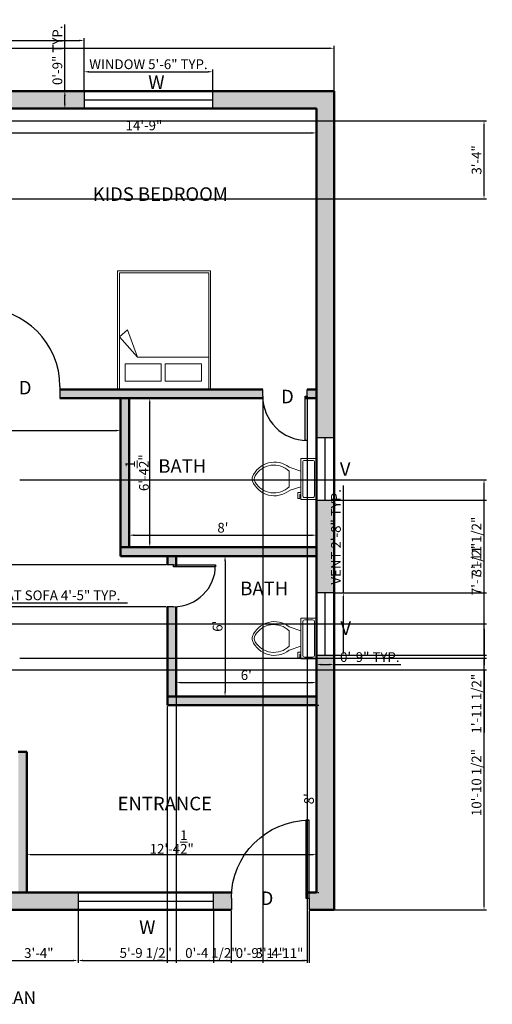
# Model space of a CAD drawing. Units: inches. Extents: x 2168 to 2706, y 2255 to 2760.
# Tile 4 of 4: x 2463 to 2706, y 2255 to 2760. Entities that reach past the tile are written whole.
import ezdxf

# ---------------------------------------------------------------- set-up
doc = ezdxf.new("R2010")
doc.units = ezdxf.units.IN
for name, color, linetype, lineweight in [('A-ANNO-DIMS', 220, 'Continuous', 18), ('A-ANNO-TEXT', 220, 'Continuous', 25), ('A-AREA-IDEN', 220, 'Continuous', 25), ('A-FLOR-FIXT', 9, 'Continuous', 18), ('A-WALL-PATT', 140, 'Continuous', 13), ('DOOR', 30, 'Continuous', 25), ('FUR', 112, 'Continuous', 18), ('WALL', 140, 'Continuous', 50), ('WINDOW', 200, 'Continuous', 25)]:
    doc.layers.add(name, color=color, linetype=linetype, lineweight=lineweight)
doc.styles.get("Standard").update_dxf_attribs({"font": 'arial.ttf'})
doc.dimstyles.new('ISO-25', dxfattribs={"dimtxt": 5, "dimasz": 2.5, "dimexe": 1.25, "dimexo": 0.625, "dimtad": 1, "dimlunit": 4, "dimtxsty": 'Standard', "dimcen": 2.5, "dimadec": 0, "dimazin": 0, "dimtfac": 1, "dimtmove": 0, "dimatfit": 3, "dimfxl": 1, "dimarcsym": 0})

# ---------------------------------------------------------------- blocks, each defined once
blk = doc.blocks.new('*U2')
for p, q in [((0, 0), (0, -6)), ((40, 0), (40, -6))]:
    blk.add_line(p, q)
blk.add_lwpolyline([(0, 0), (0, 40), (1.75, 40), (1.75, 0)], close=True)
blk.add_arc((0, 0), 40, 0, 90)
blk = doc.blocks.new('*U4')
for p, q in [((9.5, -6), (9.5, -2)), ((-10, -8.5), (-8, -8.5)), ((-10, -9.5), (-10, -8.5)), ((-7, -9.5), (-10, -9.5)), ((-8, -8.5), (-8, -8)), ((-7, -8), (-7, -9.5)), ((-4, -8), (-6, -14)), ((4, -8), (6, -14)), ((4, -14), (-4, -14))]:
    blk.add_line(p, q)
blk.add_lwpolyline([(10.5, -8), (10.5, 0), (-10.5, 0), (-10.5, -8)], close=True)
for points in [[(-9.5, -2), (-9.5, -6)], [(8.5, -1), (-8.5, -1)], [(-8.5, -7), (8.5, -7)]]:
    blk.add_lwpolyline(points)
for centre, radius, start, end in [((-8.62, -1.88), 0.884, 81.8699, 188.1301), ((8.62, -1.88), 0.884, 351.8699, 98.1301), ((-8.62, -6.12), 0.884, 171.8699, 278.1301), ((8.62, -6.12), 0.884, 261.8699, 8.1301), ((3.52, -21.58), 12.17, 141.4691, 247.9714), ((4.2, -21.82), 11.33, 136.3677, 238.9468), ((-3.52, -21.58), 12.17, 292.0284, 38.5307), ((-4.2, -21.82), 11.33, 301.053, 43.6321), ((0, -27.88), 4, 245.7318, 294.2682), ((0, -29), 4, 254.8605, 285.1395)]:
    blk.add_arc(centre, radius, start, end)
blk = doc.blocks.new('*D9')
at = {"layer": 'A-ANNO-DIMS', "color": 0, "lineweight": -2, "transparency": 16777216}
for p, q in [((2438.72, 2713.72), (2438.72, 2700.63)), ((2615.72, 2713.72), (2615.72, 2700.63)), ((2441.22, 2701.88), (2613.22, 2701.88))]:
    blk.add_line(p, q, dxfattribs=at)
at = {"layer": 'A-ANNO-DIMS', "color": 0, "transparency": 16777216}
for points in [[(2441.22, 2702.3), (2441.22, 2701.46), (2438.72, 2701.88)], [(2613.22, 2702.3), (2613.22, 2701.46), (2615.72, 2701.88)]]:
    blk.add_solid(points, dxfattribs=at)
at = {"layer": 'Defpoints', "color": 0, "transparency": 16777216}
for p in [(2438.72, 2714.35), (2615.72, 2714.35), (2615.72, 2701.88)]:
    blk.add_point(p, dxfattribs=at)
at = {"layer": 'A-ANNO-DIMS', "color": 0, "transparency": 16777216, "insert": (2527.22, 2705.06), "char_height": 5, "attachment_point": 5}
blk.add_mtext('14\'-9"', dxfattribs=at)
blk = doc.blocks.new('*D14')
at = {"layer": 'A-ANNO-DIMS', "color": 0, "lineweight": -2, "transparency": 16777216}
for p, q in [((2467.22, 2312.97), (2467.22, 2332.93)), ((2469.72, 2331.68), (2613.22, 2331.68)), ((2615.72, 2312.97), (2615.72, 2332.93))]:
    blk.add_line(p, q, dxfattribs=at)
at = {"layer": 'A-ANNO-DIMS', "color": 0, "transparency": 16777216}
for points in [[(2469.72, 2332.1), (2469.72, 2331.26), (2467.22, 2331.68)], [(2613.22, 2332.1), (2613.22, 2331.26), (2615.72, 2331.68)]]:
    blk.add_solid(points, dxfattribs=at)
at = {"layer": 'Defpoints', "color": 0, "transparency": 16777216}
for p in [(2615.72, 2331.68), (2467.22, 2312.35), (2615.72, 2312.35)]:
    blk.add_point(p, dxfattribs=at)
at = {"layer": 'A-ANNO-DIMS', "color": 0, "transparency": 16777216, "insert": (2541.47, 2338.16), "char_height": 5, "attachment_point": 5}
blk.add_mtext('12\'-4{\\H1x;\\S1/2;}"', dxfattribs=at)
blk = doc.blocks.new('*D15')
at = {"layer": 'A-ANNO-DIMS', "color": 0, "lineweight": -2, "transparency": 16777216}
for p, q in [((2615.72, 2405.85), (2615.72, 2314.85)), ((2616.35, 2408.35), (2616.97, 2408.35)), ((2616.35, 2312.35), (2616.97, 2312.35))]:
    blk.add_line(p, q, dxfattribs=at)
at = {"layer": 'A-ANNO-DIMS', "color": 0, "transparency": 16777216}
for points in [[(2615.31, 2405.85), (2616.14, 2405.85), (2615.72, 2408.35)], [(2615.31, 2314.85), (2616.14, 2314.85), (2615.72, 2312.35)]]:
    blk.add_solid(points, dxfattribs=at)
at = {"layer": 'Defpoints', "color": 0, "transparency": 16777216}
for p in [(2615.72, 2408.35), (2615.72, 2312.35), (2615.72, 2312.35)]:
    blk.add_point(p, dxfattribs=at)
at = {"layer": 'A-ANNO-DIMS', "color": 0, "transparency": 16777216, "insert": (2612.55, 2360.35), "char_height": 5, "attachment_point": 5, "rotation": 90}
blk.add_mtext("8'", dxfattribs=at)
blk = doc.blocks.new('*D16')
at = {"layer": 'A-ANNO-DIMS', "color": 0, "lineweight": -2, "transparency": 16777216}
for p, q in [((2615.1, 2484.85), (2567.58, 2484.85)), ((2568.83, 2482.35), (2568.83, 2415.35)), ((2615.1, 2412.85), (2567.58, 2412.85))]:
    blk.add_line(p, q, dxfattribs=at)
at = {"layer": 'A-ANNO-DIMS', "color": 0, "transparency": 16777216}
for points in [[(2568.42, 2482.35), (2569.25, 2482.35), (2568.83, 2484.85)], [(2568.42, 2415.35), (2569.25, 2415.35), (2568.83, 2412.85)]]:
    blk.add_solid(points, dxfattribs=at)
at = {"layer": 'Defpoints', "color": 0, "transparency": 16777216}
for p in [(2615.72, 2484.85), (2568.83, 2412.85), (2615.72, 2412.85)]:
    blk.add_point(p, dxfattribs=at)
at = {"layer": 'A-ANNO-DIMS', "color": 0, "transparency": 16777216, "insert": (2565.65, 2448.85), "char_height": 5, "attachment_point": 5, "rotation": 90}
blk.add_mtext("6'", dxfattribs=at)
blk = doc.blocks.new('*D17')
at = {"layer": 'A-ANNO-DIMS', "color": 0, "lineweight": -2, "transparency": 16777216}
for p, q in [((2543.72, 2413.47), (2543.72, 2421.19)), ((2546.22, 2419.94), (2613.22, 2419.94)), ((2615.72, 2413.47), (2615.72, 2421.19))]:
    blk.add_line(p, q, dxfattribs=at)
at = {"layer": 'A-ANNO-DIMS', "color": 0, "transparency": 16777216}
for points in [[(2546.22, 2420.36), (2546.22, 2419.53), (2543.72, 2419.94)], [(2613.22, 2420.36), (2613.22, 2419.53), (2615.72, 2419.94)]]:
    blk.add_solid(points, dxfattribs=at)
at = {"layer": 'Defpoints', "color": 0, "transparency": 16777216}
for p in [(2615.72, 2419.94), (2543.72, 2412.85), (2615.72, 2412.85)]:
    blk.add_point(p, dxfattribs=at)
at = {"layer": 'A-ANNO-DIMS', "color": 0, "transparency": 16777216, "insert": (2579.72, 2423.12), "char_height": 5, "attachment_point": 5}
blk.add_mtext("6'", dxfattribs=at)
blk = doc.blocks.new('*D18')
at = {"layer": 'A-ANNO-DIMS', "color": 0, "lineweight": -2, "transparency": 16777216}
for p, q in [((2519.72, 2489.97), (2519.72, 2496.79)), ((2522.22, 2495.54), (2613.22, 2495.54)), ((2615.72, 2489.97), (2615.72, 2496.79))]:
    blk.add_line(p, q, dxfattribs=at)
at = {"layer": 'A-ANNO-DIMS', "color": 0, "transparency": 16777216}
for points in [[(2522.22, 2495.96), (2522.22, 2495.13), (2519.72, 2495.54)], [(2613.22, 2495.96), (2613.22, 2495.13), (2615.72, 2495.54)]]:
    blk.add_solid(points, dxfattribs=at)
at = {"layer": 'Defpoints', "color": 0, "transparency": 16777216}
for p in [(2615.72, 2495.54), (2519.72, 2489.35), (2615.72, 2489.35)]:
    blk.add_point(p, dxfattribs=at)
at = {"layer": 'A-ANNO-DIMS', "color": 0, "transparency": 16777216, "insert": (2567.72, 2498.72), "char_height": 5, "attachment_point": 5}
blk.add_mtext("8'", dxfattribs=at)
blk = doc.blocks.new('*D19')
at = {"layer": 'A-ANNO-DIMS', "color": 0, "lineweight": -2, "transparency": 16777216}
for p, q in [((2520.35, 2565.85), (2531.46, 2565.85)), ((2530.21, 2491.85), (2530.21, 2563.35)), ((2520.35, 2489.35), (2531.46, 2489.35))]:
    blk.add_line(p, q, dxfattribs=at)
at = {"layer": 'A-ANNO-DIMS', "color": 0, "transparency": 16777216}
for points in [[(2529.79, 2563.35), (2530.62, 2563.35), (2530.21, 2565.85)], [(2529.79, 2491.85), (2530.62, 2491.85), (2530.21, 2489.35)]]:
    blk.add_solid(points, dxfattribs=at)
at = {"layer": 'Defpoints', "color": 0, "transparency": 16777216}
for p in [(2519.72, 2565.85), (2530.21, 2565.85), (2519.72, 2489.35)]:
    blk.add_point(p, dxfattribs=at)
at = {"layer": 'A-ANNO-DIMS', "color": 0, "transparency": 16777216, "insert": (2523.69, 2527.6), "char_height": 5, "attachment_point": 5, "rotation": 90}
blk.add_mtext('6\'-4{\\H1x;\\S1/2;}"', dxfattribs=at)
blk = doc.blocks.new('*D23')
at = {"layer": 'A-ANNO-DIMS', "color": 0, "lineweight": -2, "transparency": 16777216}
for p, q in [((2345.72, 2531.22), (2345.72, 2550.47)), ((2348.22, 2549.22), (2512.72, 2549.22)), ((2515.22, 2531.22), (2515.22, 2550.47))]:
    blk.add_line(p, q, dxfattribs=at)
at = {"layer": 'A-ANNO-DIMS', "color": 0, "transparency": 16777216}
for points in [[(2348.22, 2549.63), (2348.22, 2548.8), (2345.72, 2549.22)], [(2512.72, 2549.63), (2512.72, 2548.8), (2515.22, 2549.22)]]:
    blk.add_solid(points, dxfattribs=at)
at = {"layer": 'Defpoints', "color": 0, "transparency": 16777216}
for p in [(2515.22, 2549.22), (2345.72, 2530.6), (2515.22, 2530.6)]:
    blk.add_point(p, dxfattribs=at)
at = {"layer": 'A-ANNO-DIMS', "color": 0, "transparency": 16777216, "insert": (2430.47, 2555.69), "char_height": 5, "attachment_point": 5}
blk.add_mtext('14\'-1{\\H1x;\\S1/2;}"', dxfattribs=at)
blk = doc.blocks.new('*D29')
at = {"layer": 'A-ANNO-DIMS', "color": 0, "lineweight": -2, "transparency": 16777216}
for p, q in [((2204.72, 2723.97), (2204.72, 2746.55)), ((2207.22, 2745.3), (2622.22, 2745.3)), ((2624.72, 2723.97), (2624.72, 2746.55))]:
    blk.add_line(p, q, dxfattribs=at)
at = {"layer": 'A-ANNO-DIMS', "color": 0, "transparency": 16777216}
for points in [[(2207.22, 2745.71), (2207.22, 2744.88), (2204.72, 2745.3)], [(2622.22, 2745.71), (2622.22, 2744.88), (2624.72, 2745.3)]]:
    blk.add_solid(points, dxfattribs=at)
at = {"layer": 'Defpoints', "color": 0, "transparency": 16777216}
for p in [(2624.72, 2745.3), (2204.72, 2723.35), (2624.72, 2723.35)]:
    blk.add_point(p, dxfattribs=at)
at = {"layer": 'A-ANNO-DIMS', "color": 0, "transparency": 16777216, "insert": (2414.72, 2748.48), "char_height": 5, "attachment_point": 5}
blk.add_mtext("35'", dxfattribs=at)
blk = doc.blocks.new('BED-DOUBLE')
for p, q in [((0, 26.86), (4.14, 30.57)), ((4.14, 30.57), (9.23, 16.54)), ((9.23, 16.54), (0, 26.86)), ((45.76, 16.54), (9.23, 16.54))]:
    blk.add_line(p, q)
blk.add_lwpolyline([(46.76, 0), (46.76, 60.76), (-1, 60.76), (-1, 0)])
for points in [[(0, 0), (45.76, 0), (45.76, 59.76), (0, 59.76)], [(2.85, 4.25), (21.39, 4.25), (21.39, 13.05), (2.85, 13.05)], [(23.51, 4.25), (42.05, 4.25), (42.05, 13.05), (23.51, 13.05)]]:
    blk.add_lwpolyline(points, close=True)
blk = doc.blocks.new('WIN-66IN')
blk.add_line((0, 0), (66.01, 0))
blk.add_lwpolyline([(0, -4.5), (66.01, -4.5), (66.01, 4.5), (0, 4.5)], close=True)
blk = doc.blocks.new('VENT-32IN')
blk.add_line((0, 0), (0, 31.94))
blk.add_lwpolyline([(-4.5, 0), (4.5, 0), (4.5, 31.94), (-4.5, 31.94)], close=True)
blk = doc.blocks.new('*D40')
at = {"layer": 'A-ANNO-DIMS', "color": 0, "lineweight": -2, "transparency": 16777216}
for p, q in [((2371.67, 2453.52), (2371.67, 2462.09)), ((2374.17, 2460.84), (2422.11, 2460.84)), ((2424.61, 2453.52), (2424.61, 2462.09)), ((2424.61, 2460.84), (2518.73, 2460.84))]:
    blk.add_line(p, q, dxfattribs=at)
at = {"layer": 'A-ANNO-DIMS', "color": 0, "transparency": 16777216}
for points in [[(2374.17, 2461.26), (2374.17, 2460.43), (2371.67, 2460.84)], [(2422.11, 2461.26), (2422.11, 2460.43), (2424.61, 2460.84)]]:
    blk.add_solid(points, dxfattribs=at)
at = {"layer": 'Defpoints', "color": 0, "transparency": 16777216}
for p in [(2424.61, 2460.84), (2371.67, 2452.9), (2424.61, 2452.9)]:
    blk.add_point(p, dxfattribs=at)
at = {"layer": 'A-ANNO-DIMS', "color": 0, "transparency": 16777216, "insert": (2472.92, 2464.05), "char_height": 5, "attachment_point": 5}
blk.add_mtext('TWO-SEAT SOFA 4\'-5" TYP.', dxfattribs=at)
blk = doc.blocks.new('*D42')
at = {"layer": 'A-ANNO-DIMS', "color": 0, "lineweight": -2, "transparency": 16777216}
for p, q in [((2496.54, 2723.97), (2496.54, 2734.5)), ((2499.04, 2733.25), (2560.05, 2733.25)), ((2562.55, 2723.97), (2562.55, 2734.5))]:
    blk.add_line(p, q, dxfattribs=at)
at = {"layer": 'A-ANNO-DIMS', "color": 0, "transparency": 16777216}
for points in [[(2499.04, 2733.66), (2499.04, 2732.83), (2496.54, 2733.25)], [(2560.05, 2733.66), (2560.05, 2732.83), (2562.55, 2733.25)]]:
    blk.add_solid(points, dxfattribs=at)
at = {"layer": 'Defpoints', "color": 0, "transparency": 16777216}
for p in [(2562.55, 2733.25), (2496.54, 2723.35), (2562.55, 2723.35)]:
    blk.add_point(p, dxfattribs=at)
at = {"layer": 'A-ANNO-DIMS', "color": 0, "transparency": 16777216, "insert": (2529.55, 2736.46), "char_height": 5, "attachment_point": 5}
blk.add_mtext('WINDOW 5\'-6" TYP.', dxfattribs=at)
blk = doc.blocks.new('*D43')
at = {"layer": 'A-ANNO-DIMS', "color": 0, "lineweight": -2, "transparency": 16777216}
for p, q in [((2486.64, 2723.35), (2486.64, 2757.57)), ((2495.92, 2723.35), (2485.39, 2723.35)), ((2486.64, 2716.85), (2486.64, 2720.85)), ((2495.92, 2714.35), (2485.39, 2714.35))]:
    blk.add_line(p, q, dxfattribs=at)
at = {"layer": 'A-ANNO-DIMS', "color": 0, "transparency": 16777216}
for points in [[(2486.22, 2720.85), (2487.06, 2720.85), (2486.64, 2723.35)], [(2486.22, 2716.85), (2487.06, 2716.85), (2486.64, 2714.35)]]:
    blk.add_solid(points, dxfattribs=at)
at = {"layer": 'Defpoints', "color": 0, "transparency": 16777216}
for p in [(2486.64, 2723.35), (2496.54, 2723.35), (2496.54, 2714.35)]:
    blk.add_point(p, dxfattribs=at)
at = {"layer": 'A-ANNO-DIMS', "color": 0, "transparency": 16777216, "insert": (2483.46, 2741.71), "char_height": 5, "attachment_point": 5, "rotation": 90}
blk.add_mtext('0\'-9" TYP.', dxfattribs=at)
blk = doc.blocks.new('*D44')
at = {"layer": 'A-ANNO-DIMS', "color": 0, "lineweight": -2, "transparency": 16777216}
for p, q in [((2629.51, 2465.92), (2629.51, 2520.98)), ((2625.35, 2465.92), (2630.76, 2465.92)), ((2629.51, 2436.48), (2629.51, 2463.42)), ((2625.35, 2433.98), (2630.76, 2433.98))]:
    blk.add_line(p, q, dxfattribs=at)
at = {"layer": 'A-ANNO-DIMS', "color": 0, "transparency": 16777216}
for points in [[(2629.1, 2463.42), (2629.93, 2463.42), (2629.51, 2465.92)], [(2629.1, 2436.48), (2629.93, 2436.48), (2629.51, 2433.98)]]:
    blk.add_solid(points, dxfattribs=at)
at = {"layer": 'Defpoints', "color": 0, "transparency": 16777216}
for p in [(2624.72, 2465.92), (2629.51, 2465.92), (2624.72, 2433.98)]:
    blk.add_point(p, dxfattribs=at)
at = {"layer": 'A-ANNO-DIMS', "color": 0, "transparency": 16777216, "insert": (2626.34, 2494.7), "char_height": 5, "attachment_point": 5, "rotation": 90}
blk.add_mtext('VENT 2\'-8" TYP.', dxfattribs=at)
blk = doc.blocks.new('*D45')
at = {"layer": 'A-ANNO-DIMS', "color": 0, "lineweight": -2, "transparency": 16777216}
for p, q in [((2615.72, 2433.36), (2615.72, 2427.94)), ((2624.72, 2433.36), (2624.72, 2427.94)), ((2618.22, 2429.19), (2622.22, 2429.19)), ((2624.72, 2429.19), (2658.95, 2429.19))]:
    blk.add_line(p, q, dxfattribs=at)
at = {"layer": 'A-ANNO-DIMS', "color": 0, "transparency": 16777216}
for points in [[(2618.22, 2429.61), (2618.22, 2428.77), (2615.72, 2429.19)], [(2622.22, 2429.61), (2622.22, 2428.77), (2624.72, 2429.19)]]:
    blk.add_solid(points, dxfattribs=at)
at = {"layer": 'Defpoints', "color": 0, "transparency": 16777216}
for p in [(2615.72, 2433.98), (2624.72, 2433.98), (2624.72, 2429.19)]:
    blk.add_point(p, dxfattribs=at)
at = {"layer": 'A-ANNO-DIMS', "color": 0, "transparency": 16777216, "insert": (2643.09, 2432.37), "char_height": 5, "attachment_point": 5}
blk.add_mtext('0\'-9" TYP.', dxfattribs=at)
blk = doc.blocks.new('*D46')
at = {"layer": 'A-ANNO-DIMS', "color": 0, "lineweight": -2, "transparency": 16777216}
for p, q in [((2572.05, 2302.72), (2572.05, 2276.15)), ((2612.05, 2302.72), (2612.05, 2276.15)), ((2574.55, 2277.4), (2609.55, 2277.4))]:
    blk.add_line(p, q, dxfattribs=at)
at = {"layer": 'A-ANNO-DIMS', "color": 0, "transparency": 16777216}
for points in [[(2574.55, 2277.81), (2574.55, 2276.98), (2572.05, 2277.4)], [(2609.55, 2277.81), (2609.55, 2276.98), (2612.05, 2277.4)]]:
    blk.add_solid(points, dxfattribs=at)
at = {"layer": 'Defpoints', "color": 0, "transparency": 16777216}
for p in [(2572.05, 2303.35), (2612.05, 2303.35), (2612.05, 2277.4)]:
    blk.add_point(p, dxfattribs=at)
at = {"layer": 'A-ANNO-DIMS', "color": 0, "transparency": 16777216, "insert": (2592.05, 2280.58), "char_height": 5, "attachment_point": 5}
blk.add_mtext('3\'-4"', dxfattribs=at)
blk = doc.blocks.new('*D48')
at = {"layer": 'A-ANNO-DIMS', "color": 0, "lineweight": -2, "transparency": 16777216}
for p, q in [((2543.72, 2412.22), (2543.72, 2276.15)), ((2539.22, 2407.72), (2539.22, 2276.15)), ((2536.72, 2277.4), (2534.22, 2277.4)), ((2539.22, 2277.4), (2543.72, 2277.4)), ((2546.22, 2277.4), (2574.92, 2277.4))]:
    blk.add_line(p, q, dxfattribs=at)
at = {"layer": 'A-ANNO-DIMS', "color": 0, "transparency": 16777216}
for points in [[(2536.72, 2277.81), (2536.72, 2276.98), (2539.22, 2277.4)], [(2546.22, 2277.81), (2546.22, 2276.98), (2543.72, 2277.4)]]:
    blk.add_solid(points, dxfattribs=at)
at = {"layer": 'Defpoints', "color": 0, "transparency": 16777216}
for p in [(2543.72, 2412.85), (2539.22, 2408.35), (2543.72, 2277.4)]:
    blk.add_point(p, dxfattribs=at)
at = {"layer": 'A-ANNO-DIMS', "color": 0, "transparency": 16777216, "insert": (2561.82, 2280.61), "char_height": 5, "attachment_point": 5}
blk.add_mtext('0\'-4 1/2"', dxfattribs=at)
blk = doc.blocks.new('*D50')
at = {"layer": 'A-ANNO-DIMS', "color": 0, "lineweight": -2, "transparency": 16777216}
for p, q in [((2610.95, 2566.3), (2610.95, 2276.15)), ((2588.18, 2565.22), (2588.18, 2276.15)), ((2590.68, 2277.4), (2608.45, 2277.4))]:
    blk.add_line(p, q, dxfattribs=at)
at = {"layer": 'A-ANNO-DIMS', "color": 0, "transparency": 16777216}
for points in [[(2590.68, 2277.81), (2590.68, 2276.98), (2588.18, 2277.4)], [(2608.45, 2277.81), (2608.45, 2276.98), (2610.95, 2277.4)]]:
    blk.add_solid(points, dxfattribs=at)
at = {"layer": 'Defpoints', "color": 0, "transparency": 16777216}
for p in [(2588.18, 2565.85), (2610.95, 2566.93), (2610.95, 2277.4)]:
    blk.add_point(p, dxfattribs=at)
at = {"layer": 'A-ANNO-DIMS', "color": 0, "transparency": 16777216, "insert": (2599.56, 2280.53), "char_height": 5, "attachment_point": 5}
blk.add_mtext('1\'-11"', dxfattribs=at)
blk = doc.blocks.new('*D51')
at = {"layer": 'A-ANNO-DIMS', "color": 0, "lineweight": -2, "transparency": 16777216}
for p, q in [((2178.77, 2480.31), (2178.77, 2508.53)), ((2538.6, 2480.31), (2177.52, 2480.31)), ((2178.77, 2461.31), (2178.77, 2477.81)), ((2538.6, 2458.81), (2177.52, 2458.81))]:
    blk.add_line(p, q, dxfattribs=at)
at = {"layer": 'A-ANNO-DIMS', "color": 0, "transparency": 16777216}
for points in [[(2178.36, 2477.81), (2179.19, 2477.81), (2178.77, 2480.31)], [(2178.36, 2461.31), (2179.19, 2461.31), (2178.77, 2458.81)]]:
    blk.add_solid(points, dxfattribs=at)
at = {"layer": 'Defpoints', "color": 0, "transparency": 16777216}
for p in [(2178.77, 2480.31), (2539.22, 2480.31), (2539.22, 2458.81)]:
    blk.add_point(p, dxfattribs=at)
at = {"layer": 'A-ANNO-DIMS', "color": 0, "transparency": 16777216, "insert": (2175.56, 2495.67), "char_height": 5, "attachment_point": 5, "rotation": 90}
blk.add_mtext('1\'-9 1/2"', dxfattribs=at)
blk = doc.blocks.new('*D52')
at = {"layer": 'A-ANNO-DIMS', "color": 0, "lineweight": -2, "transparency": 16777216}
for p, q in [((2463.6, 2523.98), (2702.92, 2523.98)), ((2701.67, 2434.92), (2701.67, 2521.48)), ((2463.6, 2432.42), (2702.92, 2432.42))]:
    blk.add_line(p, q, dxfattribs=at)
at = {"layer": 'A-ANNO-DIMS', "color": 0, "transparency": 16777216}
for points in [[(2701.26, 2521.48), (2702.09, 2521.48), (2701.67, 2523.98)], [(2701.26, 2434.92), (2702.09, 2434.92), (2701.67, 2432.42)]]:
    blk.add_solid(points, dxfattribs=at)
at = {"layer": 'Defpoints', "color": 0, "transparency": 16777216}
for p in [(2462.98, 2523.98), (2701.67, 2523.98), (2462.98, 2432.42)]:
    blk.add_point(p, dxfattribs=at)
at = {"layer": 'A-ANNO-DIMS', "color": 0, "transparency": 16777216, "insert": (2698.46, 2478.2), "char_height": 5, "attachment_point": 5, "rotation": 90}
blk.add_mtext('7\'-7 1/2"', dxfattribs=at)
blk = doc.blocks.new('*D55')
at = {"layer": 'A-ANNO-DIMS', "color": 0, "lineweight": -2, "transparency": 16777216}
for p, q in [((2299.9, 2450), (2702.92, 2450)), ((2701.67, 2447.5), (2701.67, 2428.92)), ((2299.9, 2426.42), (2702.92, 2426.42)), ((2701.67, 2426.42), (2701.67, 2394.31))]:
    blk.add_line(p, q, dxfattribs=at)
at = {"layer": 'A-ANNO-DIMS', "color": 0, "transparency": 16777216}
for points in [[(2701.26, 2447.5), (2702.09, 2447.5), (2701.67, 2450)], [(2701.26, 2428.92), (2702.09, 2428.92), (2701.67, 2426.42)]]:
    blk.add_solid(points, dxfattribs=at)
at = {"layer": 'Defpoints', "color": 0, "transparency": 16777216}
for p in [(2299.27, 2450), (2299.27, 2426.42), (2701.67, 2426.42)]:
    blk.add_point(p, dxfattribs=at)
at = {"layer": 'A-ANNO-DIMS', "color": 0, "transparency": 16777216, "insert": (2698.46, 2409.11), "char_height": 5, "attachment_point": 5, "rotation": 90}
blk.add_mtext('1\'-11 1/2"', dxfattribs=at)
blk = doc.blocks.new('*D61')
at = {"layer": 'A-ANNO-DIMS', "color": 0, "lineweight": -2, "transparency": 16777216}
for p, q in [((2453.21, 2302.72), (2453.21, 2276.15)), ((2493.42, 2302.72), (2493.42, 2276.15)), ((2455.71, 2277.4), (2490.92, 2277.4))]:
    blk.add_line(p, q, dxfattribs=at)
at = {"layer": 'A-ANNO-DIMS', "color": 0, "transparency": 16777216}
for points in [[(2455.71, 2277.81), (2455.71, 2276.98), (2453.21, 2277.4)], [(2490.92, 2277.81), (2490.92, 2276.98), (2493.42, 2277.4)]]:
    blk.add_solid(points, dxfattribs=at)
at = {"layer": 'Defpoints', "color": 0, "transparency": 16777216}
for p in [(2453.21, 2303.35), (2493.42, 2303.35), (2493.42, 2277.4)]:
    blk.add_point(p, dxfattribs=at)
at = {"layer": 'A-ANNO-DIMS', "color": 0, "transparency": 16777216, "insert": (2473.31, 2280.58), "char_height": 5, "attachment_point": 5}
blk.add_mtext('3\'-4"', dxfattribs=at)
blk = doc.blocks.new('*D62')
at = {"layer": 'A-ANNO-DIMS', "color": 0, "lineweight": -2, "transparency": 16777216}
for p, q in [((2493.42, 2302.72), (2493.42, 2276.15)), ((2562.88, 2302.72), (2562.88, 2276.15)), ((2495.92, 2277.4), (2560.38, 2277.4))]:
    blk.add_line(p, q, dxfattribs=at)
at = {"layer": 'A-ANNO-DIMS', "color": 0, "transparency": 16777216}
for points in [[(2495.92, 2277.81), (2495.92, 2276.98), (2493.42, 2277.4)], [(2560.38, 2277.81), (2560.38, 2276.98), (2562.88, 2277.4)]]:
    blk.add_solid(points, dxfattribs=at)
at = {"layer": 'Defpoints', "color": 0, "transparency": 16777216}
for p in [(2493.42, 2303.35), (2562.88, 2303.35), (2562.88, 2277.4)]:
    blk.add_point(p, dxfattribs=at)
at = {"layer": 'A-ANNO-DIMS', "color": 0, "transparency": 16777216, "insert": (2528.15, 2280.61), "char_height": 5, "attachment_point": 5}
blk.add_mtext('5\'-9 1/2"', dxfattribs=at)
blk = doc.blocks.new('*D63')
at = {"layer": 'A-ANNO-DIMS', "color": 0, "lineweight": -2, "transparency": 16777216}
for p, q in [((2562.88, 2302.72), (2562.88, 2276.15)), ((2572.05, 2302.72), (2572.05, 2276.15)), ((2565.38, 2277.4), (2569.55, 2277.4)), ((2572.05, 2277.4), (2589.09, 2277.4))]:
    blk.add_line(p, q, dxfattribs=at)
at = {"layer": 'A-ANNO-DIMS', "color": 0, "transparency": 16777216}
for points in [[(2565.38, 2277.81), (2565.38, 2276.98), (2562.88, 2277.4)], [(2569.55, 2277.81), (2569.55, 2276.98), (2572.05, 2277.4)]]:
    blk.add_solid(points, dxfattribs=at)
at = {"layer": 'Defpoints', "color": 0, "transparency": 16777216}
for p in [(2562.88, 2303.35), (2572.05, 2303.35), (2572.05, 2277.4)]:
    blk.add_point(p, dxfattribs=at)
at = {"layer": 'A-ANNO-DIMS', "color": 0, "transparency": 16777216, "insert": (2581.82, 2280.57), "char_height": 5, "attachment_point": 5}
blk.add_mtext('0\'-9"', dxfattribs=at)
blk = doc.blocks.new('*D65')
at = {"layer": 'A-ANNO-DIMS', "color": 0, "lineweight": -2, "transparency": 16777216}
for p, q in [((2396.13, 2723.97), (2396.13, 2750.55)), ((2398.63, 2749.3), (2494.04, 2749.3)), ((2496.54, 2723.97), (2496.54, 2750.55))]:
    blk.add_line(p, q, dxfattribs=at)
at = {"layer": 'A-ANNO-DIMS', "color": 0, "transparency": 16777216}
for points in [[(2398.63, 2749.71), (2398.63, 2748.88), (2396.13, 2749.3)], [(2494.04, 2749.71), (2494.04, 2748.88), (2496.54, 2749.3)]]:
    blk.add_solid(points, dxfattribs=at)
at = {"layer": 'Defpoints', "color": 0, "transparency": 16777216}
for p in [(2496.54, 2749.3), (2396.13, 2723.35), (2496.54, 2723.35)]:
    blk.add_point(p, dxfattribs=at)
at = {"layer": 'A-ANNO-DIMS', "color": 0, "transparency": 16777216, "insert": (2446.33, 2752.51), "char_height": 5, "attachment_point": 5}
blk.add_mtext('8\'-4 1/2"', dxfattribs=at)
blk = doc.blocks.new('*D72')
at = {"layer": 'A-ANNO-DIMS', "color": 0, "lineweight": -2, "transparency": 16777216}
for p, q in [((2625.35, 2433.98), (2702.92, 2433.98)), ((2701.67, 2305.85), (2701.67, 2431.48)), ((2625.35, 2303.35), (2702.92, 2303.35))]:
    blk.add_line(p, q, dxfattribs=at)
at = {"layer": 'A-ANNO-DIMS', "color": 0, "transparency": 16777216}
for points in [[(2701.26, 2431.48), (2702.09, 2431.48), (2701.67, 2433.98)], [(2701.26, 2305.85), (2702.09, 2305.85), (2701.67, 2303.35)]]:
    blk.add_solid(points, dxfattribs=at)
at = {"layer": 'Defpoints', "color": 0, "transparency": 16777216}
for p in [(2624.72, 2433.98), (2701.67, 2433.98), (2624.72, 2303.35)]:
    blk.add_point(p, dxfattribs=at)
at = {"layer": 'A-ANNO-DIMS', "color": 0, "transparency": 16777216, "insert": (2698.46, 2368.66), "char_height": 5, "attachment_point": 5, "rotation": 90}
blk.add_mtext('10\'-10 1/2"', dxfattribs=at)
blk = doc.blocks.new('*D73')
at = {"layer": 'A-ANNO-DIMS', "color": 0, "lineweight": -2, "transparency": 16777216}
for p, q in [((2625.35, 2513.51), (2702.92, 2513.51)), ((2701.67, 2468.42), (2701.67, 2511.01)), ((2625.35, 2465.92), (2702.92, 2465.92))]:
    blk.add_line(p, q, dxfattribs=at)
at = {"layer": 'A-ANNO-DIMS', "color": 0, "transparency": 16777216}
for points in [[(2701.26, 2511.01), (2702.09, 2511.01), (2701.67, 2513.51)], [(2701.26, 2468.42), (2702.09, 2468.42), (2701.67, 2465.92)]]:
    blk.add_solid(points, dxfattribs=at)
at = {"layer": 'Defpoints', "color": 0, "transparency": 16777216}
for p in [(2624.72, 2513.51), (2701.67, 2513.51), (2624.72, 2465.92)]:
    blk.add_point(p, dxfattribs=at)
at = {"layer": 'A-ANNO-DIMS', "color": 0, "transparency": 16777216, "insert": (2698.46, 2489.71), "char_height": 5, "attachment_point": 5, "rotation": 90}
blk.add_mtext('3\'-11 1/2"', dxfattribs=at)
blk = doc.blocks.new('*D77')
at = {"layer": 'A-ANNO-DIMS', "color": 0, "lineweight": -2, "transparency": 16777216}
for p, q in [((2290.85, 2708.02), (2702.92, 2708.02)), ((2701.67, 2670.52), (2701.67, 2705.52)), ((2290.85, 2668.02), (2702.92, 2668.02))]:
    blk.add_line(p, q, dxfattribs=at)
at = {"layer": 'A-ANNO-DIMS', "color": 0, "transparency": 16777216}
for points in [[(2701.26, 2705.52), (2702.09, 2705.52), (2701.67, 2708.02)], [(2701.26, 2670.52), (2702.09, 2670.52), (2701.67, 2668.02)]]:
    blk.add_solid(points, dxfattribs=at)
at = {"layer": 'Defpoints', "color": 0, "transparency": 16777216}
for p in [(2290.22, 2708.02), (2701.67, 2708.02), (2290.22, 2668.02)]:
    blk.add_point(p, dxfattribs=at)
at = {"layer": 'A-ANNO-DIMS', "color": 0, "transparency": 16777216, "insert": (2698.49, 2688.02), "char_height": 5, "attachment_point": 5, "rotation": 90}
blk.add_mtext('3\'-4"', dxfattribs=at)

msp = doc.modelspace()

# ---------------------------------------------------------------- hatches: boundary and pattern name
at = {"layer": 'A-WALL-PATT'}
h = msp.add_hatch(color=256, dxfattribs=at)
h.dxf.hatch_style = 1
h.paths.add_polyline_path([(2330.12, 2723.347), (2204.724, 2723.347), (2204.724, 2662.147), (2213.724, 2662.147), (2213.724, 2714.347), (2285.724, 2714.347), (2330.12, 2714.347)])
h.paths.add_polyline_path([(2496.542, 2723.347), (2396.128, 2723.347), (2396.128, 2714.347), (2434.224, 2714.347), (2496.542, 2714.347)])
h.paths.add_polyline_path([(2624.724, 2723.347), (2562.55, 2723.347), (2562.55, 2714.347), (2615.724, 2714.347), (2615.724, 2545.448), (2624.724, 2545.448)])
h.paths.add_polyline_path([(2438.724, 2714.347), (2434.224, 2714.347), (2434.224, 2570.347), (2426.591, 2570.347), (2426.591, 2565.847), (2438.724, 2565.847), (2444.149, 2565.847), (2444.149, 2570.347), (2438.724, 2570.347)])
h.paths.add_polyline_path([(2290.224, 2668.023), (2285.724, 2668.023), (2285.724, 2570.347), (2213.724, 2570.347), (2213.724, 2565.847), (2290.224, 2565.847), (2386.591, 2565.847), (2386.591, 2570.347), (2290.224, 2570.347)])
h.paths.add_polyline_path([(2514.678, 2570.347), (2514.678, 2630.11), (2560.439, 2630.11), (2560.439, 2570.347)], flags=16)
h.paths.add_polyline_path([(2517.528, 2574.595), (2517.528, 2583.399), (2536.063, 2583.399), (2536.063, 2574.595)], flags=0)
h.paths.add_polyline_path([(2523.909, 2586.89), (2514.678, 2597.212), (2518.822, 2600.918)], flags=0)
h.paths.add_polyline_path([(2538.189, 2574.595), (2538.189, 2583.399), (2556.724, 2583.399), (2556.724, 2574.595)], flags=0)
h.paths.add_polyline_path([(2560.439, 2630.11), (2560.439, 2570.347), (2514.678, 2570.347), (2514.678, 2630.11)])
h.paths.add_polyline_path([(2213.724, 2389.588), (2204.724, 2389.588), (2204.724, 2303.347), (2229.06, 2303.347), (2229.06, 2312.347), (2213.724, 2312.347)])
h.paths.add_polyline_path([(2213.724, 2507.677), (2204.724, 2507.677), (2204.724, 2462.696), (2213.724, 2462.696)])
h.paths.add_polyline_path([(2204.724, 2553.759), (2213.724, 2553.759), (2213.724, 2613.731), (2204.724, 2613.731)])
h = msp.add_hatch(color=256, dxfattribs=at)
h.dxf.hatch_style = 1
h.paths.add_polyline_path([(2318.775, 2312.347), (2295.068, 2312.347), (2295.068, 2303.347), (2318.775, 2303.347)])
h.paths.add_polyline_path([(2403.851, 2312.347), (2390.724, 2312.347), (2384.782, 2312.347), (2384.782, 2303.347), (2403.851, 2303.347)])
h.paths.add_polyline_path([(2390.724, 2384.347), (2390.724, 2388.847), (2383.783, 2388.847), (2383.783, 2384.347), (2386.224, 2384.347), (2386.224, 2312.347), (2390.724, 2312.347), (2390.724, 2324.834)])
h.paths.add_polyline_path([(2493.418, 2312.347), (2467.224, 2312.347), (2453.211, 2312.347), (2453.211, 2303.347), (2493.418, 2303.347)])
h.paths.add_polyline_path([(2467.224, 2384.347), (2462.724, 2384.347), (2462.724, 2312.347), (2467.224, 2312.347)])
h.paths.add_polyline_path([(2572.054, 2309.347, -0.0187698), (2572.166, 2312.347), (2562.881, 2312.347), (2562.881, 2303.347), (2572.054, 2303.347)])
h.paths.add_polyline_path([(2624.724, 2433.98), (2615.724, 2433.98), (2615.724, 2432.059), (2615.724, 2412.847), (2615.724, 2312.347), (2612.054, 2312.347), (2612.054, 2309.347), (2612.054, 2303.347), (2624.724, 2303.347)])
h.paths.add_polyline_path([(2543.724, 2452.016), (2543.724, 2458.843, -0.0148288), (2542.449, 2458.805), (2539.224, 2458.805), (2539.224, 2452.016), (2539.224, 2412.847), (2543.724, 2412.847)])
h.paths.add_polyline_path([(2615.724, 2412.847), (2543.724, 2412.847), (2539.224, 2412.847), (2539.224, 2408.347), (2615.724, 2408.347)])
h.paths.add_polyline_path([(2624.724, 2513.509), (2615.724, 2513.509), (2615.724, 2465.92), (2624.724, 2465.92)])
h.paths.add_polyline_path([(2588.15, 2570.347), (2484.149, 2570.347), (2484.149, 2565.847), (2588.176, 2565.847, -0.0118396), (2588.15, 2566.926)])
h.paths.add_polyline_path([(2615.724, 2570.347), (2610.953, 2570.347), (2610.953, 2566.926), (2610.953, 2565.847), (2615.724, 2565.847)])
h.paths.add_polyline_path([(2519.724, 2565.847), (2515.224, 2565.847), (2515.224, 2489.347), (2519.724, 2489.347)])
h.paths.add_polyline_path([(2615.724, 2489.347), (2519.724, 2489.347), (2515.224, 2489.347), (2515.224, 2484.847), (2615.724, 2484.847)])
h.paths.add_polyline_path([(2543.724, 2484.847), (2539.224, 2484.847), (2539.224, 2480.308), (2542.449, 2480.308), (2543.724, 2480.308)])

# ---------------------------------------------------------------- linework, layer by layer
at = {"layer": 'WALL'}
for p, q in [((2204.724, 2723.347), (2624.724, 2723.347)), ((2624.724, 2723.347), (2624.724, 2303.347)), ((2484.149, 2570.347), (2588.15, 2570.347)), ((2484.149, 2565.847), (2588.176, 2565.847)), ((2515.224, 2484.847), (2515.224, 2565.847)), ((2519.724, 2489.347), (2519.724, 2565.847)), ((2609.956, 2565.847), (2615.724, 2565.847)), ((2610.953, 2570.347), (2615.724, 2570.347)), ((2615.724, 2412.847), (2615.724, 2565.847)), ((2519.724, 2489.347), (2515.224, 2489.347)), ((2615.724, 2484.847), (2515.224, 2484.847)), ((2615.724, 2489.347), (2519.724, 2489.347)), ((2539.224, 2480.308), (2539.224, 2484.847)), ((2543.724, 2479.367), (2543.724, 2484.847)), ((2539.224, 2452.016), (2539.224, 2458.805)), ((2543.724, 2452.016), (2543.724, 2458.843)), ((2539.224, 2412.847), (2539.224, 2452.016)), ((2543.724, 2412.847), (2543.724, 2452.016)), ((2539.224, 2412.847), (2615.724, 2412.847)), ((2539.224, 2412.847), (2539.224, 2408.347)), ((2615.724, 2412.847), (2543.724, 2412.847)), ((2539.224, 2408.347), (2615.724, 2408.347)), ((2462.724, 2384.347), (2467.224, 2384.347)), ((2467.224, 2384.347), (2467.224, 2312.347)), ((2467.224, 2312.347), (2467.224, 2384.347)), ((2467.224, 2312.347), (2572.166, 2312.347)), ((2610.304, 2312.347), (2611.224, 2312.347)), ((2572.054, 2303.347), (2204.724, 2303.347)), ((2624.724, 2303.347), (2612.054, 2303.347))]:
    msp.add_line(p, q, dxfattribs=at)
for points in [[(2572.054, 2303.347), (2204.724, 2303.347), (2204.724, 2723.347), (2624.724, 2723.347), (2624.724, 2303.347), (2612.054, 2303.347)], [(2572.166, 2312.347), (2213.724, 2312.347), (2213.724, 2714.347), (2615.724, 2714.347), (2615.724, 2312.347), (2610.304, 2312.347)]]:
    msp.add_lwpolyline(points, dxfattribs=at)
at = {"layer": 'WINDOW'}
msp.add_line((2493.418, 2307.847), (2562.881, 2307.847), dxfattribs=at)
msp.add_lwpolyline([(2493.418, 2303.347), (2562.881, 2303.347), (2562.881, 2312.347), (2493.418, 2312.347)], close=True, dxfattribs=at)

# ---------------------------------------------------------------- block references
at = {"layer": 'A-FLOR-FIXT', "xscale": -1, "rotation": 270}
for p in [(2615.724, 2524.383), (2615.724, 2442.559)]:
    msp.add_blockref('*U4', p, dxfattribs=at)
at = {"layer": 'DOOR'}
msp.add_blockref('*U2', (2444.149, 2571.847), dxfattribs=at)
for p, xscale, yscale, zscale, rotation in [((2610.953, 2566.926), 0.5700860826601627, 0.5700860826601627, 0.5700860826601627, 180), ((2542.449, 2480.308), 0.5375669162669471, 0.5375669162669471, 0.5375669162669471, 270)]:
    msp.add_blockref('*U2', p, dxfattribs=dict(at, xscale=xscale, yscale=yscale, zscale=zscale, rotation=rotation))
at = {"layer": 'DOOR', "xscale": -1}
msp.add_blockref('*U2', (2612.054, 2309.347), dxfattribs=at)
at = {"layer": 'FUR'}
msp.add_blockref('BED-DOUBLE', (2514.678, 2570.347), dxfattribs=at)
at = {"layer": 'WINDOW'}
for name, p in [('WIN-66IN', (2496.542, 2718.847)), ('VENT-32IN', (2620.224, 2513.509)), ('VENT-32IN', (2620.224, 2433.98))]:
    msp.add_blockref(name, p, dxfattribs=at)

# ---------------------------------------------------------------- texts
at = {"layer": 'A-ANNO-TEXT', "attachment_point": 1}
for s, width, gutter_width, insert, char_height in [('W', 121.01281, 34.753, (2529.444, 2731.347), 6.951), ('D', 121.01281, 34.753, (2463.045, 2574.701), 6.951), ('D', 121.01281, 34.753, (2597.58, 2570.14), 6.951), ('V', 121.01281, 34.753, (2627.711, 2532.994), 6.951), ('V', 121.01281, 34.753, (2628.005, 2451.328), 6.951), ('D', 121.01281, 34.753, (2587.094, 2312.785), 6.951), ('W', 121.01281, 34.753, (2524.779, 2297.922), 6.951), ('GROUND FLOOR PLAN', 655.2644, 32.568, (2379.787, 2261.546), 6.51363)]:
    msp.add_mtext_dynamic_manual_height_columns(s, width=width, gutter_width=gutter_width, heights=[0], dxfattribs=dict(at, insert=insert, char_height=char_height))
at = {"layer": 'A-AREA-IDEN', "attachment_point": 1}
for s, insert, char_height in [('KIDS BEDROOM', (2500.945, 2673.974), 6.95057), ('BATH', (2534.589, 2534.495), 6.9506), ('BATH', (2576.634, 2471.706), 6.9506), ('ENTRANCE', (2513.725, 2361.36), 6.9506)]:
    msp.add_mtext_dynamic_manual_height_columns(s, width=121.01281, gutter_width=34.753, heights=[0], dxfattribs=dict(at, insert=insert, char_height=char_height))

# ---------------------------------------------------------------- dimensions: what is measured, and where the dimension line sits
at = {"layer": 'A-ANNO-DIMS'}
for base, p1, p2, override, picture, middle in [((2496.542, 2749.297), (2396.128, 2723.347), (2496.542, 2723.347), {"dimdec": 1, "dimlfac": 1, "dimrnd": 0, "dimzin": 1, "dimdsep": 46, "dimlunit": 4, "dimfrac": 2}, '*D65', (2446.335, 2752.507)), ((2624.724, 2745.296), (2204.724, 2723.347), (2624.724, 2723.347), {"dimclrd": 0, "dimclre": 0, "dimclrt": 0}, '*D29', (2414.724, 2748.475)), ((2615.724, 2701.881), (2438.724, 2714.347), (2615.724, 2714.347), {"dimclrd": 0, "dimclre": 0, "dimclrt": 0}, '*D9', (2527.224, 2705.059)), ((2610.953, 2277.397), (2588.176, 2565.847), (2610.953, 2566.926), {"dimdec": 1, "dimlfac": 1, "dimrnd": 0, "dimzin": 1, "dimdsep": 46, "dimlunit": 4, "dimfrac": 2}, '*D50', (2599.564, 2280.532)), ((2515.224, 2549.215), (2345.724, 2530.597), (2515.224, 2530.597), {"dimclrd": 0, "dimclre": 0, "dimclrt": 0}, '*D23', (2430.474, 2555.694)), ((2615.724, 2495.542), (2519.724, 2489.347), (2615.724, 2489.347), {"dimclrd": 0, "dimclre": 0, "dimclrt": 0}, '*D18', (2567.724, 2498.72)), ((2615.724, 2419.942), (2543.724, 2412.847), (2615.724, 2412.847), {"dimclrd": 0, "dimclre": 0, "dimclrt": 0}, '*D17', (2579.724, 2423.12)), ((2543.724, 2277.397), (2539.224, 2408.347), (2543.724, 2412.847), {"dimdec": 1, "dimlfac": 1, "dimrnd": 0, "dimzin": 1, "dimdsep": 46, "dimlunit": 4, "dimfrac": 2}, '*D48', (2561.82, 2280.607)), ((2615.724, 2331.681), (2467.224, 2312.347), (2615.724, 2312.347), {"dimclrd": 0, "dimclre": 0, "dimclrt": 0}, '*D14', (2541.474, 2338.16)), ((2493.418, 2277.397), (2453.211, 2303.347), (2493.418, 2303.347), {"dimdec": 1, "dimlfac": 1, "dimrnd": 0, "dimzin": 1, "dimdsep": 46, "dimlunit": 4, "dimfrac": 2}, '*D61', (2473.315, 2280.577)), ((2562.881, 2277.397), (2493.418, 2303.347), (2562.881, 2303.347), {"dimdec": 1, "dimlfac": 1, "dimrnd": 0, "dimzin": 1, "dimdsep": 46, "dimlunit": 4, "dimfrac": 2}, '*D62', (2528.15, 2280.607)), ((2572.054, 2277.397), (2562.881, 2303.347), (2572.054, 2303.347), {"dimdec": 1, "dimlfac": 1, "dimrnd": 0, "dimzin": 1, "dimdsep": 46, "dimlunit": 4, "dimfrac": 2}, '*D63', (2581.824, 2280.575)), ((2612.054, 2277.397), (2572.054, 2303.347), (2612.054, 2303.347), {"dimdec": 1, "dimlfac": 1, "dimrnd": 0, "dimzin": 1, "dimdsep": 46, "dimlunit": 4, "dimfrac": 2}, '*D46', (2592.054, 2280.577))]:
    dim = msp.add_linear_dim(base=base, p1=p1, p2=p2, dimstyle='ISO-25', override=override, dxfattribs=at)
    dim.commit()
    dim.dimension.update_dxf_attribs({"geometry": picture, "text_midpoint": middle})
for base, p1, p2, text, picture, middle in [((2486.641, 2723.347), (2496.542, 2714.347), (2496.542, 2723.347), '<> TYP.', '*D43', (2483.463, 2741.711)), ((2629.515, 2465.92), (2624.724, 2433.98), (2624.724, 2465.92), 'VENT <> TYP.', '*D44', (2626.337, 2494.698))]:
    dim = msp.add_linear_dim(base=base, p1=p1, p2=p2, angle=90, text=text, dimstyle='ISO-25', override={"dimdec": 1, "dimlfac": 1, "dimrnd": 0, "dimzin": 1, "dimdsep": 46, "dimlunit": 4, "dimfrac": 2}, dxfattribs=at)
    dim.commit()
    dim.dimension.update_dxf_attribs({"geometry": picture, "text_midpoint": middle})
for base, p1, p2, text, picture, middle in [((2562.55, 2733.248), (2496.542, 2723.347), (2562.55, 2723.347), 'WINDOW <> TYP.', '*D42', (2529.546, 2736.46)), ((2424.614, 2460.842), (2371.666, 2452.9), (2424.614, 2452.9), 'TWO-SEAT SOFA <> TYP.', '*D40', (2472.922, 2464.054)), ((2624.724, 2429.189), (2615.724, 2433.98), (2624.724, 2433.98), '<> TYP.', '*D45', (2643.088, 2432.367))]:
    dim = msp.add_linear_dim(base=base, p1=p1, p2=p2, text=text, dimstyle='ISO-25', override={"dimdec": 1, "dimlfac": 1, "dimrnd": 0, "dimzin": 1, "dimdsep": 46, "dimlunit": 4, "dimfrac": 2}, dxfattribs=at)
    dim.commit()
    dim.dimension.update_dxf_attribs({"geometry": picture, "text_midpoint": middle})
for base, p1, p2, override, picture, middle in [((2701.674, 2708.023), (2290.224, 2668.023), (2290.224, 2708.023), {"dimdec": 1, "dimlfac": 1, "dimrnd": 0, "dimzin": 1, "dimdsep": 46, "dimlunit": 4, "dimfrac": 2}, '*D77', (2698.494, 2688.023)), ((2530.207, 2565.847), (2519.724, 2489.347), (2519.724, 2565.847), {"dimclrd": 0, "dimclre": 0, "dimclrt": 0}, '*D19', (2523.685, 2527.597)), ((2701.674, 2523.979), (2462.979, 2432.42), (2462.979, 2523.979), {"dimdec": 1, "dimlfac": 1, "dimrnd": 0, "dimzin": 1, "dimdsep": 46, "dimlunit": 4, "dimfrac": 2}, '*D52', (2698.464, 2478.199)), ((2701.674, 2513.509), (2624.724, 2465.92), (2624.724, 2513.509), {"dimdec": 1, "dimlfac": 1, "dimrnd": 0, "dimzin": 1, "dimdsep": 46, "dimlunit": 4, "dimfrac": 2}, '*D73', (2698.462, 2489.714)), ((2178.774, 2480.308), (2539.224, 2458.805), (2539.224, 2480.308), {"dimdec": 1, "dimlfac": 1, "dimrnd": 0, "dimzin": 1, "dimdsep": 46, "dimlunit": 4, "dimfrac": 2}, '*D51', (2175.564, 2495.669)), ((2568.832, 2412.847), (2615.724, 2484.847), (2615.724, 2412.847), {"dimclrd": 0, "dimclre": 0, "dimclrt": 0}, '*D16', (2565.654, 2448.847)), ((2701.674, 2426.417), (2299.272, 2449.996), (2299.272, 2426.417), {"dimdec": 1, "dimlfac": 1, "dimrnd": 0, "dimzin": 1, "dimdsep": 46, "dimlunit": 4, "dimfrac": 2}, '*D55', (2698.464, 2409.114)), ((2701.674, 2433.98), (2624.724, 2303.347), (2624.724, 2433.98), {"dimdec": 1, "dimlfac": 1, "dimrnd": 0, "dimzin": 1, "dimdsep": 46, "dimlunit": 4, "dimfrac": 2}, '*D72', (2698.464, 2368.664)), ((2615.724, 2312.347), (2615.724, 2408.347), (2615.724, 2312.347), {"dimclrd": 0, "dimclre": 0, "dimclrt": 0}, '*D15', (2612.546, 2360.347))]:
    dim = msp.add_linear_dim(base=base, p1=p1, p2=p2, angle=90, dimstyle='ISO-25', override=override, dxfattribs=at)
    dim.commit()
    dim.dimension.update_dxf_attribs({"geometry": picture, "text_midpoint": middle})

doc.saveas('drawing.dxf')
